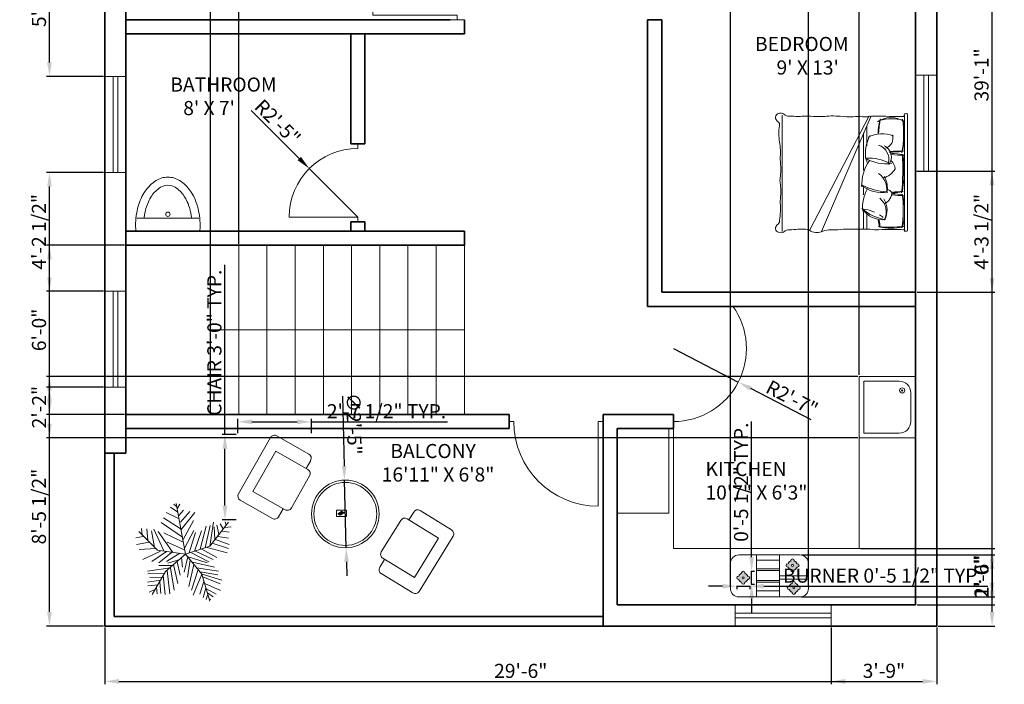
# Model space of a CAD drawing. Units: inches. Extents: x 88375 to 88815, y 24230 to 25146.
# Tile 1 of 3: x 88375 to 88794, y 24230 to 24513. Entities that reach past the tile are written whole.
import ezdxf

# ---------------------------------------------------------------- set-up
doc = ezdxf.new("R2010")
doc.units = ezdxf.units.IN
for name, color, linetype, lineweight in [('A-ANNO-DIMS', 2, 'Continuous', 18), ('A-AREA-IDEN', 7, 'Continuous', 18), ('A-EQPM', 4, 'Continuous', 18), ('A-FLOR-CASE', 7, 'Continuous', 18), ('A-FLOR-STRS', 7, 'Continuous', 18), ('A-WALL', 7, 'Continuous', 35), ('doors', 50, 'Continuous', 18), ('L-PLNT', 7, 'Continuous', 13), ('SANTEH', 5, 'Continuous', 18), ('windows', 70, 'Continuous', 18)]:
    doc.layers.add(name, color=color, linetype=linetype, lineweight=lineweight)
doc.layers.add('A-FURN', color=141, linetype='Continuous', lineweight=18, true_color=0xadddf7)
doc.layers.add('A-FURN-PATT', color=141, linetype='Continuous', lineweight=13, true_color=0xadddf7)
doc.styles.get("Standard").update_dxf_attribs({"font": 'arial.ttf'})
doc.dimstyles.new('ISO-25', dxfattribs={"dimtxt": 6, "dimasz": 6, "dimexe": 1.25, "dimexo": 0.625, "dimtad": 1, "dimdec": 0, "dimlunit": 3, "dimtxsty": 'Standard', "dimcen": 2.5, "dimclrd": 1, "dimclre": 1, "dimclrt": 2, "dimadec": 0, "dimazin": 0, "dimtfac": 1, "dimtdec": 0, "dimtmove": 0, "dimatfit": 3, "dimfxl": 1, "dimarcsym": 0})

# ---------------------------------------------------------------- blocks, each defined once
blk = doc.blocks.new('Trees - Imperial')
for p, q in [((-10.186, 53.64), (-13.084, 55.962)), ((0, 0), (-10.5, 57)), ((-9.099, 51.782), (-6.563, 55.962)), ((-7.288, 39.707), (-21.778, 46.673)), ((-8.737, 47.138), (-17.069, 52.711)), ((-7.65, 43.423), (-2.578, 49.46)), ((-5.839, 35.992), (4.667, 48.067)), ((-5.114, 27.632), (10.463, 46.673)), ((-3.665, 19.273), (-27.574, 35.527)), ((-5.114, 28.097), (-24.676, 40.636)), ((-2.941, 16.486), (8.652, 37.85)), ((27, 9), (48, 36)), ((27.127, 9.056), (31.112, 35.992)), ((38.719, 34.134), (41.979, 28.561)), ((44.153, 36.456), (45.239, 32.741)), ((-31.5, 4.5), (-52.5, 25.5)), ((-48.585, 21.131), (-49.309, 29.026)), ((-43.513, 28.561), (-42.427, 15.558)), ((-38.442, 26.239), (-34.819, 7.663)), ((-35.544, 28.097), (-24.314, 3.947)), ((-14.533, 2.09), (-30.834, 25.31)), ((-24.314, 23.917), (-2.941, 13.7)), ((-1.129, 6.734), (9.014, 26.704)), ((3.942, 1.625), (11.187, 24.381)), ((10.101, 3.483), (17.708, 26.239)), ((16.259, 5.805), (23.142, 31.348)), ((22.055, 7.198), (27.489, 32.277)), ((31.836, 30.883), (32.561, 16.486)), ((35.096, 32.741), (37.27, 22.524)), ((40.53, 25.775), (48.862, 24.846)), ((43.791, 29.954), (51.036, 30.883)), ((-47.498, 19.737), (-55.83, 18.344)), ((-40.615, 13.7), (-55.105, 10.913)), ((-20.691, 13.7), (-1.129, 4.876)), ((29.662, 12.307), (48.137, 6.269)), ((33.285, 16.486), (48.862, 10.913)), ((36.183, 19.737), (48.137, 17.88)), ((-33.37, 6.269), (-52.207, 5.34)), ((-28.299, 3.483), (-47.86, -5.805)), ((-21.416, 3.018), (-38.079, -8.128)), ((0, 0), (-31.5, 4.5)), ((-15.982, 2.09), (-30.11, -9.521)), ((0, 0), (-22.5, -19.5)), ((-6.563, 1.161), (-21.416, -8.128)), ((0, 0), (27, 9)), ((0, 0), (18, -22.5)), ((6.478, 1.625), (26.04, -8.592)), ((11.187, 3.483), (30.749, -5.805)), ((18.07, 5.805), (35.096, -3.483)), ((24.229, 7.663), (46.688, 1.625)), ((-6.563, -5.805), (-19.967, -9.985)), ((-9.461, -8.592), (-6.201, -23.453)), ((-4.752, -3.483), (-3.665, -14.629)), ((2.493, -3.019), (-1.491, -20.202)), ((1.769, -2.555), (24.229, -9.521)), ((5.029, -6.27), (2.131, -25.775)), ((7.565, -9.056), (32.198, -14.629)), ((-17.431, -15.094), (-42.789, -18.809)), ((-24.314, -21.596), (-42.427, -22.06)), ((-22.5, -19.5), (-37.5, -45)), ((-15.257, -12.772), (-30.11, -12.772)), ((-20.691, -18.345), (-17.793, -44.352)), ((-17.069, -15.094), (-12.721, -40.172)), ((-13.446, -11.378), (-8.737, -32.741)), ((9.014, -11.378), (3.58, -35.992)), ((14.085, -16.951), (6.478, -40.172)), ((12.274, -15.094), (36.907, -18.809)), ((16.259, -19.738), (36.183, -22.989)), ((-28.299, -29.026), (-42.789, -31.348)), ((-26.849, -26.24), (-40.253, -25.775)), ((-29.023, -30.884), (-27.936, -43.887)), ((-25.038, -23.918), (-22.865, -45.281)), ((18.07, -22.524), (8.289, -45.745)), ((20.244, -30.419), (15.897, -44.816)), ((18, -22.5), (27, -52.5)), ((18.433, -22.524), (40.53, -29.026)), ((19.157, -25.311), (38.719, -33.206)), ((21.331, -32.741), (39.081, -40.636)), ((-30.834, -34.135), (-42.427, -35.528)), ((-34.457, -39.708), (-40.978, -42.494)), ((-32.646, -36.921), (-31.921, -44.352)), ((22.78, -37.85), (19.519, -48.532)), ((22.78, -38.314), (34.372, -44.816)), ((24.591, -43.423), (30.749, -47.603)), ((24.591, -45.745), (23.142, -50.854)), ((26.764, -49.925), (28.213, -50.854))]:
    blk.add_line(p, q)
blk = doc.blocks.new('BED-DOUBLE-PLAN')
for p, q in [((1.4, 0.9), (1.4, 50.31)), ((15.52, 1.15), (36.6, 50.31)), ((53.33, 0.9), (53.33, 50.31)), ((16.31, 1.15), (41.56, 49.64)), ((17.42, 42.88), (17.42, 49.34)), ((18.75, 41.86), (18.75, 49.34)), ((18.75, 31.74), (18.75, 34.71)), ((18.75, 8.33), (18.75, 24.37)), ((17.42, 19.9), (17.42, 20.88)), ((17.42, 5.64), (17.42, 13.88))]:
    blk.add_line(p, q)
blk.add_lwpolyline([(1.54, 49.41, 0.098699), (1.25, 50.08, 0.222522), (0, 50.08), (0, 0.33, 0.171621), (1.3, 0.3, 0.102495), (1.54, 1.48, 0.015571), (6.35, 1.41, 0.00267), (12.35, 1.29, 0.058958), (15.95, 1.46, -0.038458), (19.2, 1.53, 0.025508), (23.25, 1.53, -0.039412), (28.66, 1.33, 0.016498), (32.6, 1.18, -0.035771), (40.08, 1.43, 0.045388), (45.04, 1.29, -0.080578), (47.62, 1.41, 0.026504), (50.99, 1.23, -0.211134), (52.07, 0.79, 0.329446), (55.35, 0.34, 0.37589), (56.22, 2.29, 0.123892), (55.14, 3.69, -0.342539), (54.6, 5.33, 0.07104), (54.53, 12.17, -0.036442), (54.14, 15.72, -0.046791), (54.19, 18.58, 0.023628), (54.14, 21.2, -0.055897), (54.2, 27.56, 0.053528), (54.38, 28.63, 0.053528), (54.2, 29.69, -0.055897), (54.14, 36.05, 0.026973), (54.19, 38.35, -0.036947), (54.14, 41.97, -0.036442), (54.53, 45.52, -0.281256), (55.14, 47.2, -0.521995), (55.14, 47.2, 0.123892), (56.22, 48.6, 0.37589), (55.35, 50.55, 0.329446), (52.07, 50.1, -0.211134), (50.99, 49.66, 0.026504), (47.62, 49.48, -0.06219), (44.27, 49.36, -0.218233), (41.22, 50.22, 0.123513), (38.6, 50.78, 0.129887), (36.08, 50.23, -0.095063), (32.6, 49.71, 0.016498), (28.66, 49.56, -0.039412), (23.25, 49.36, 0.025508), (19.2, 49.36, -0.038458), (15.95, 49.43, 0.058958), (12.35, 49.6, 0.00267), (6.35, 49.48, 0.015571)], format="xyb", close=True)
for centre, radius, start, end in [((28.69, 41.4), 27.41, 165.0181, 193.7392), ((7.34, -1.74), 50.25, 84.0935, 96.4707), ((54.72, 40.85), 52.84, 171.3714, 186.917), ((6.88, 26.06), 22.91, 77.3175, 101.7435), ((30.71, 48.94), 18.95, 180.6432, 190.2707), ((-1.93, 44.06), 14.51, 5.447, 17.4199), ((17.81, 41.21), 9.06, 151.6404, 211.3345), ((16.4, 41.97), 7.31, 151.8876, 231.8707), ((10.64, 34.91), 10.43, 32.3262, 97), ((7.31, 27.91), 17.47, 47.3201, 81.4624), ((20.44, 56.37), 15.6, 229.9508, 236.951), ((20.44, 56.37), 15.6, 246.2982, 263.8539), ((12.85, 33.14), 6.24, 118.1996, 176.5061), ((2.46, 40.16), 16.73, 330.9467, 5.467), ((2.85, 15.46), 19.59, 79.1667, 93.123), ((2.68, 52.73), 19.37, 267.8261, 281.4767), ((6.96, 53.59), 19.33, 255.3434, 268.3876), ((106.24, 23.67), 104.16, 174.3658, 183.3969), ((7.12, 7.71), 26.2, 91.8337, 100.6945), ((8.83, 34.94), 2.36, 210.1134, 265.8974), ((10.93, 20.25), 13.55, 49.1339, 100.5299), ((18.11, 31.85), 9.49, 168.4081, 212.0077), ((56.67, 24.77), 55.1, 170.934, 187.4266), ((17.21, 32.51), 8.35, 173.5607, 234.2853), ((8.19, 10.11), 23.35, 61.605, 88.1749), ((2.96, 30.11), 16.53, 323.2201, 4.4972), ((12.63, 19.42), 8.48, 105.4018, 149.7122), ((11.01, 24.39), 5.75, 186.8992, 226.0421), ((9.41, 5.14), 16.41, 58.6542, 99.1977), ((12.4, 18.76), 5.47, 144.1671, 243.8421), ((16.24, 36.43), 17.32, 241.0456, 274.1497), ((14.48, 19.78), 6.53, 168.0413, 250.8342), ((2.41, -6.96), 24.84, 79.589, 92.0447), ((43.42, 8.57), 41.72, 168.5485, 188.3029), ((6.97, 44.4), 27.2, 259.5301, 269.934), ((1.41, 17.17), 16.55, 332.3859, 9.8951), ((35.22, 9.22), 33.81, 168.0142, 190.5125), ((1.64, 92.63), 76.52, 270.1063, 274.3312), ((7.34, -22.96), 39.54, 89.1536, 97.5533), ((10.98, 10.47), 4.74, 108.9387, 194.6725), ((10.84, 22.26), 13.47, 249.3026, 296.5026), ((274.44, -22.62), 263.89, 173.2132, 174.5476), ((-20.26, 9.91), 32.87, 348.1169, 357.8849), ((7.08, 12.11), 10.21, 237.51, 303.8336), ((6.79, 19.75), 17.39, 253.9263, 287.1409)]:
    blk.add_arc(centre, radius, start, end)
blk = doc.blocks.new('CHAIR-BALCONY')
for p, q in [((13.87, 34.67), (0.26, 10.71)), ((30.23, 27.65), (16.56, 35.41)), ((6.37, 11.76), (16.1, 28.88)), ((29.8, 21.1), (16.1, 28.88)), ((30.97, 24.96), (29.02, 21.54)), ((22.76, 4.72), (30.53, 18.41)), ((6.37, 11.76), (20.07, 3.98)), ((6.37, 11.76), (20.07, 3.98)), ((14.67, 0.26), (1, 8.02)), ((17.35, 1), (19.3, 4.42))]:
    blk.add_line(p, q)
for centre, start, end in [((15.58, 33.7), 60.3989, 150.3989), ((29.25, 25.94), 330.3989, 60.3989), ((28.82, 19.39), 330.3989, 60.3989), ((1.97, 9.73), 150.3989, 240.3989), ((21.04, 5.69), 240.3989, 330.3989), ((15.64, 1.97), 240.3989, 330.3989)]:
    blk.add_arc(centre, 1.97, start, end)
blk = doc.blocks.new('WINDOW-PLAN-WIDE')
for p, q in [((3.5, 40.79), (3.5, 0)), ((5.5, 40.79), (5.5, 0))]:
    blk.add_line(p, q)
blk.add_lwpolyline([(0, 0), (9, 0), (9, 40.79), (0, 40.79)], close=True)
blk = doc.blocks.new('DOOR-SWING-36IN')
for p, q in [((3, 38), (3, 40)), ((3, 0), (3, 2)), ((3, 2), (39, 2)), ((6, 0), (0, 0))]:
    blk.add_line(p, q)
blk.add_arc((3, 2), 36, 0, 90)
blk = doc.blocks.new('COOKTOP-BURNER')
h = blk.add_hatch(color=256)
h.dxf.hatch_style = 1
h.paths.add_polyline_path([(3.49, 4.67), (3.49, 4.81, 1), (2.04, 4.81), (2.04, 4.67, 0.214506), (0.86, 3.49), (0.72, 3.49, 1), (0.72, 2.04), (0.86, 2.04, 0.214506), (2.04, 0.86), (2.04, 0.72, 1), (3.49, 0.72), (3.49, 0.86, 0.214506), (4.67, 2.04), (4.81, 2.04, 1), (4.81, 3.49), (4.67, 3.49, 0.214506)])
h.paths.add_polyline_path([(3.21, 2.77, -1), (2.32, 2.77, -1)], flags=16)
for p, q in [((2.04, 4.81), (2.04, 4.67)), ((3.49, 4.81), (3.49, 4.67)), ((0.72, 3.49), (0.86, 3.49)), ((0.72, 2.04), (0.86, 2.04)), ((2.04, 0.86), (2.04, 0.72)), ((3.49, 0.86), (3.49, 0.72)), ((4.67, 3.49), (4.81, 3.49)), ((4.67, 2.04), (4.81, 2.04))]:
    blk.add_line(p, q)
blk.add_circle((2.77, 2.77), 0.442)
for centre, radius, start, end in [((2.77, 2.77), 2.04, 110.7864, 159.2136), ((2.77, 4.81), 0.724, 0, 180), ((2.77, 2.77), 2.04, 20.7864, 69.2136), ((0.72, 2.77), 0.724, 90, 270), ((2.77, 2.77), 2.04, 200.7864, 249.2136), ((2.77, 0.72), 0.724, 180, 0), ((2.77, 2.77), 2.04, 290.7864, 339.2136), ((4.81, 2.77), 0.724, 270, 90)]:
    blk.add_arc(centre, radius, start, end)
blk = doc.blocks.new('*D23')
at = {"layer": 'A-ANNO-DIMS', "color": 1, "lineweight": -2, "transparency": 16777216}
for p, q in [((88674.45, 24271.96), (88668.45, 24271.96)), ((88680.45, 24272.16), (88680.45, 24270.71)), ((88680.45, 24271.96), (88685.98, 24271.96)), ((88685.98, 24272.16), (88685.98, 24270.71)), ((88691.98, 24271.96), (88787.24, 24271.96))]:
    blk.add_line(p, q, dxfattribs=at)
at = {"layer": 'A-ANNO-DIMS', "color": 1, "transparency": 16777216}
for points in [[(88674.45, 24272.96), (88674.45, 24270.96), (88680.45, 24271.96)], [(88691.98, 24272.96), (88691.98, 24270.96), (88685.98, 24271.96)]]:
    blk.add_solid(points, dxfattribs=at)
at = {"layer": 'Defpoints', "color": 0, "transparency": 16777216}
for p in [(88680.45, 24272.79), (88685.98, 24272.79), (88685.98, 24271.96)]:
    blk.add_point(p, dxfattribs=at)
at = {"layer": 'A-ANNO-DIMS', "color": 2, "transparency": 16777216, "insert": (88742.61, 24275.69), "char_height": 6, "attachment_point": 5}
blk.add_mtext('BURNER 0\'-5 1/2" TYP.', dxfattribs=at)
blk = doc.blocks.new('*D24')
at = {"layer": 'A-ANNO-DIMS', "color": 1, "lineweight": -2, "transparency": 16777216}
for p, q in [((88686.8, 24284.32), (88686.8, 24342.12)), ((88686.6, 24278.32), (88688.05, 24278.32)), ((88686.8, 24272.79), (88686.8, 24278.32)), ((88686.6, 24272.79), (88688.05, 24272.79)), ((88686.8, 24266.79), (88686.8, 24260.79))]:
    blk.add_line(p, q, dxfattribs=at)
at = {"layer": 'A-ANNO-DIMS', "color": 1, "transparency": 16777216}
for points in [[(88685.8, 24284.32), (88687.8, 24284.32), (88686.8, 24278.32)], [(88685.8, 24266.79), (88687.8, 24266.79), (88686.8, 24272.79)]]:
    blk.add_solid(points, dxfattribs=at)
at = {"layer": 'Defpoints', "color": 0, "transparency": 16777216}
for p in [(88685.98, 24278.32), (88686.8, 24278.32), (88685.98, 24272.79)]:
    blk.add_point(p, dxfattribs=at)
at = {"layer": 'A-ANNO-DIMS', "color": 2, "transparency": 16777216, "insert": (88683.08, 24316.22), "char_height": 6, "attachment_point": 5, "rotation": 90}
blk.add_mtext('0\'-5 1/2" TYP.', dxfattribs=at)
blk = doc.blocks.new('*D27')
at = {"layer": 'A-ANNO-DIMS', "color": 1, "lineweight": -2, "transparency": 16777216}
for p, q in [((88462.68, 24336.49), (88462.68, 24408.65)), ((88467.49, 24336.49), (88461.43, 24336.49)), ((88462.68, 24306.26), (88462.68, 24330.49)), ((88467.49, 24300.26), (88461.43, 24300.26))]:
    blk.add_line(p, q, dxfattribs=at)
at = {"layer": 'A-ANNO-DIMS', "color": 1, "transparency": 16777216}
for points in [[(88461.68, 24330.49), (88463.68, 24330.49), (88462.68, 24336.49)], [(88461.68, 24306.26), (88463.68, 24306.26), (88462.68, 24300.26)]]:
    blk.add_solid(points, dxfattribs=at)
at = {"layer": 'Defpoints', "color": 0, "transparency": 16777216}
for p in [(88462.68, 24336.49), (88468.12, 24336.49), (88468.12, 24300.26)]:
    blk.add_point(p, dxfattribs=at)
at = {"layer": 'A-ANNO-DIMS', "color": 2, "transparency": 16777216, "insert": (88458.95, 24375.57), "char_height": 6, "attachment_point": 5, "rotation": 90}
blk.add_mtext('CHAIR 3\'-0" TYP.', dxfattribs=at)
blk = doc.blocks.new('*D28')
at = {"layer": 'A-ANNO-DIMS', "color": 1, "lineweight": -2, "transparency": 16777216}
for p, q in [((88468.12, 24337.11), (88468.12, 24343.17)), ((88474.12, 24341.92), (88493.47, 24341.92)), ((88499.47, 24337.11), (88499.47, 24343.17)), ((88499.47, 24341.92), (88557.38, 24341.92))]:
    blk.add_line(p, q, dxfattribs=at)
at = {"layer": 'A-ANNO-DIMS', "color": 1, "transparency": 16777216}
for points in [[(88474.12, 24342.92), (88474.12, 24340.92), (88468.12, 24341.92)], [(88493.47, 24342.92), (88493.47, 24340.92), (88499.47, 24341.92)]]:
    blk.add_solid(points, dxfattribs=at)
at = {"layer": 'Defpoints', "color": 0, "transparency": 16777216}
for p in [(88499.47, 24341.92), (88468.12, 24336.49), (88499.47, 24336.49)]:
    blk.add_point(p, dxfattribs=at)
at = {"layer": 'A-ANNO-DIMS', "color": 2, "transparency": 16777216, "insert": (88531.43, 24345.65), "char_height": 6, "attachment_point": 5}
blk.add_mtext('2\'-7 1/2" TYP.', dxfattribs=at)
blk = doc.blocks.new('*D33')
at = {"layer": 'A-ANNO-DIMS', "color": 1, "lineweight": -2, "transparency": 16777216}
for p, q in [((88411.55, 24254.4), (88411.55, 24230.22)), ((88765.55, 24254.4), (88765.55, 24230.22)), ((88417.55, 24231.47), (88759.55, 24231.47))]:
    blk.add_line(p, q, dxfattribs=at)
at = {"layer": 'A-ANNO-DIMS', "color": 1, "transparency": 16777216}
for points in [[(88417.55, 24232.47), (88417.55, 24230.47), (88411.55, 24231.47)], [(88759.55, 24232.47), (88759.55, 24230.47), (88765.55, 24231.47)]]:
    blk.add_solid(points, dxfattribs=at)
at = {"layer": 'Defpoints', "color": 0, "transparency": 16777216}
for p in [(88411.55, 24255.02), (88765.55, 24255.02), (88765.55, 24231.47)]:
    blk.add_point(p, dxfattribs=at)
at = {"layer": 'A-ANNO-DIMS', "color": 2, "transparency": 16777216, "insert": (88588.55, 24235.16), "char_height": 6, "attachment_point": 5}
blk.add_mtext('29\'-6"', dxfattribs=at)
blk = doc.blocks.new('*D34')
at = {"layer": 'A-ANNO-DIMS', "color": 1, "lineweight": -2, "transparency": 16777216}
for p, q in [((88766.18, 24724.02), (88790.35, 24724.02)), ((88789.1, 24261.02), (88789.1, 24718.02)), ((88766.18, 24255.02), (88790.35, 24255.02))]:
    blk.add_line(p, q, dxfattribs=at)
at = {"layer": 'A-ANNO-DIMS', "color": 1, "transparency": 16777216}
for points in [[(88788.1, 24718.02), (88790.1, 24718.02), (88789.1, 24724.02)], [(88788.1, 24261.02), (88790.1, 24261.02), (88789.1, 24255.02)]]:
    blk.add_solid(points, dxfattribs=at)
at = {"layer": 'Defpoints', "color": 0, "transparency": 16777216}
for p in [(88765.55, 24724.02), (88789.1, 24724.02), (88765.55, 24255.02)]:
    blk.add_point(p, dxfattribs=at)
at = {"layer": 'A-ANNO-DIMS', "color": 2, "transparency": 16777216, "insert": (88785.41, 24489.52), "char_height": 6, "attachment_point": 5, "rotation": 90}
blk.add_mtext('39\'-1"', dxfattribs=at)
blk = doc.blocks.new('*D37')
at = {"layer": 'A-ANNO-DIMS', "color": 1, "lineweight": -2, "transparency": 16777216}
for p, q in [((88757.18, 24448.59), (88790.35, 24448.59)), ((88789.1, 24403.02), (88789.1, 24442.59)), ((88757.18, 24397.02), (88790.35, 24397.02))]:
    blk.add_line(p, q, dxfattribs=at)
at = {"layer": 'A-ANNO-DIMS', "color": 1, "transparency": 16777216}
for points in [[(88788.1, 24442.59), (88790.1, 24442.59), (88789.1, 24448.59)], [(88788.1, 24403.02), (88790.1, 24403.02), (88789.1, 24397.02)]]:
    blk.add_solid(points, dxfattribs=at)
at = {"layer": 'Defpoints', "color": 0, "transparency": 16777216}
for p in [(88756.55, 24448.59), (88789.1, 24448.59), (88756.55, 24397.02)]:
    blk.add_point(p, dxfattribs=at)
at = {"layer": 'A-ANNO-DIMS', "color": 2, "transparency": 16777216, "insert": (88785.37, 24422.81), "char_height": 6, "attachment_point": 5, "rotation": 90}
blk.add_mtext('4\'-3 1/2"', dxfattribs=at)
blk = doc.blocks.new('*D39')
at = {"layer": 'A-ANNO-DIMS', "color": 1, "lineweight": -2, "transparency": 16777216}
for p, q in [((88410.93, 24356.67), (88386.75, 24356.67)), ((88388, 24261.02), (88388, 24350.67)), ((88410.93, 24255.02), (88386.75, 24255.02))]:
    blk.add_line(p, q, dxfattribs=at)
at = {"layer": 'A-ANNO-DIMS', "color": 1, "transparency": 16777216}
for points in [[(88387, 24350.67), (88389, 24350.67), (88388, 24356.67)], [(88387, 24261.02), (88389, 24261.02), (88388, 24255.02)]]:
    blk.add_solid(points, dxfattribs=at)
at = {"layer": 'Defpoints', "color": 0, "transparency": 16777216}
for p in [(88388, 24356.67), (88411.55, 24356.67), (88411.55, 24255.02)]:
    blk.add_point(p, dxfattribs=at)
at = {"layer": 'A-ANNO-DIMS', "color": 2, "transparency": 16777216, "insert": (88384.28, 24305.85), "char_height": 6, "attachment_point": 5, "rotation": 90}
blk.add_mtext('8\'-5 1/2"', dxfattribs=at)
blk = doc.blocks.new('*D40')
at = {"layer": 'A-ANNO-DIMS', "color": 1, "lineweight": -2, "transparency": 16777216}
for p, q in [((88410.93, 24448.05), (88386.75, 24448.05)), ((88388, 24403.46), (88388, 24442.05)), ((88410.93, 24397.46), (88386.75, 24397.46))]:
    blk.add_line(p, q, dxfattribs=at)
at = {"layer": 'A-ANNO-DIMS', "color": 1, "transparency": 16777216}
for points in [[(88387, 24442.05), (88389, 24442.05), (88388, 24448.05)], [(88387, 24403.46), (88389, 24403.46), (88388, 24397.46)]]:
    blk.add_solid(points, dxfattribs=at)
at = {"layer": 'Defpoints', "color": 0, "transparency": 16777216}
for p in [(88388, 24448.05), (88411.55, 24448.05), (88411.55, 24397.46)]:
    blk.add_point(p, dxfattribs=at)
at = {"layer": 'A-ANNO-DIMS', "color": 2, "transparency": 16777216, "insert": (88384.28, 24422.76), "char_height": 6, "attachment_point": 5, "rotation": 90}
blk.add_mtext('4\'-2 1/2"', dxfattribs=at)
blk = doc.blocks.new('*D41')
at = {"layer": 'A-ANNO-DIMS', "color": 1, "lineweight": -2, "transparency": 16777216}
for p, q in [((88410.93, 24549.01), (88386.75, 24549.01)), ((88388, 24494.84), (88388, 24543.01)), ((88410.93, 24488.84), (88386.75, 24488.84))]:
    blk.add_line(p, q, dxfattribs=at)
at = {"layer": 'A-ANNO-DIMS', "color": 1, "transparency": 16777216}
for points in [[(88387, 24543.01), (88389, 24543.01), (88388, 24549.01)], [(88387, 24494.84), (88389, 24494.84), (88388, 24488.84)]]:
    blk.add_solid(points, dxfattribs=at)
at = {"layer": 'Defpoints', "color": 0, "transparency": 16777216}
for p in [(88388, 24549.01), (88411.55, 24549.01), (88411.55, 24488.84)]:
    blk.add_point(p, dxfattribs=at)
at = {"layer": 'A-ANNO-DIMS', "color": 2, "transparency": 16777216, "insert": (88384.31, 24518.92), "char_height": 6, "attachment_point": 5, "rotation": 90}
blk.add_mtext('5\'-0"', dxfattribs=at)
blk = doc.blocks.new('*D42')
at = {"layer": 'A-ANNO-DIMS', "color": 1, "lineweight": -2, "transparency": 16777216}
for p, q in [((88720.63, 24254.4), (88720.63, 24230.22)), ((88765.55, 24254.4), (88765.55, 24230.22)), ((88726.63, 24231.47), (88759.55, 24231.47))]:
    blk.add_line(p, q, dxfattribs=at)
at = {"layer": 'A-ANNO-DIMS', "color": 1, "transparency": 16777216}
for points in [[(88726.63, 24232.47), (88726.63, 24230.47), (88720.63, 24231.47)], [(88759.55, 24232.47), (88759.55, 24230.47), (88765.55, 24231.47)]]:
    blk.add_solid(points, dxfattribs=at)
at = {"layer": 'Defpoints', "color": 0, "transparency": 16777216}
for p in [(88720.63, 24255.02), (88765.55, 24255.02), (88765.55, 24231.47)]:
    blk.add_point(p, dxfattribs=at)
at = {"layer": 'A-ANNO-DIMS', "color": 2, "transparency": 16777216, "insert": (88743.09, 24235.16), "char_height": 6, "attachment_point": 5}
blk.add_mtext('3\'-9"', dxfattribs=at)
blk = doc.blocks.new('*D43')
at = {"layer": 'A-ANNO-DIMS', "color": 1, "lineweight": -2, "transparency": 16777216}
for p, q in [((88420.55, 24345.65), (88420.55, 24748.82)), ((88426.55, 24747.57), (88450.55, 24747.57)), ((88456.55, 24345.65), (88456.55, 24748.82))]:
    blk.add_line(p, q, dxfattribs=at)
at = {"layer": 'A-ANNO-DIMS', "color": 1, "transparency": 16777216}
for points in [[(88426.55, 24748.57), (88426.55, 24746.57), (88420.55, 24747.57)], [(88450.55, 24748.57), (88450.55, 24746.57), (88456.55, 24747.57)]]:
    blk.add_solid(points, dxfattribs=at)
at = {"layer": 'Defpoints', "color": 0, "transparency": 16777216}
for p in [(88456.55, 24747.57), (88420.55, 24345.02), (88456.55, 24345.02)]:
    blk.add_point(p, dxfattribs=at)
at = {"layer": 'A-ANNO-DIMS', "color": 2, "transparency": 16777216, "insert": (88438.55, 24751.26), "char_height": 6, "attachment_point": 5}
blk.add_mtext('3\'-0"', dxfattribs=at)
blk = doc.blocks.new('*D44')
at = {"layer": 'A-ANNO-DIMS', "color": 1, "lineweight": -2, "transparency": 16777216}
for p, q in [((88419.93, 24417.02), (88386.75, 24417.02)), ((88388, 24351.02), (88388, 24411.02)), ((88419.93, 24345.02), (88386.75, 24345.02))]:
    blk.add_line(p, q, dxfattribs=at)
at = {"layer": 'A-ANNO-DIMS', "color": 1, "transparency": 16777216}
for points in [[(88387, 24411.02), (88389, 24411.02), (88388, 24417.02)], [(88387, 24351.02), (88389, 24351.02), (88388, 24345.02)]]:
    blk.add_solid(points, dxfattribs=at)
at = {"layer": 'Defpoints', "color": 0, "transparency": 16777216}
for p in [(88388, 24417.02), (88420.55, 24417.02), (88420.55, 24345.02)]:
    blk.add_point(p, dxfattribs=at)
at = {"layer": 'A-ANNO-DIMS', "color": 2, "transparency": 16777216, "insert": (88384.31, 24381.02), "char_height": 6, "attachment_point": 5, "rotation": 90}
blk.add_mtext('6\'-0"', dxfattribs=at)
blk = doc.blocks.new('*D45')
at = {"layer": 'A-ANNO-DIMS', "color": 1, "lineweight": -2, "transparency": 16777216}
for p, q in [((88450.55, 24747.57), (88444.55, 24747.57)), ((88456.55, 24417.65), (88456.55, 24748.82)), ((88456.55, 24747.57), (88468.55, 24747.57)), ((88468.55, 24417.65), (88468.55, 24748.82)), ((88474.55, 24747.57), (88497.19, 24747.57))]:
    blk.add_line(p, q, dxfattribs=at)
at = {"layer": 'A-ANNO-DIMS', "color": 1, "transparency": 16777216}
for points in [[(88450.55, 24748.57), (88450.55, 24746.57), (88456.55, 24747.57)], [(88474.55, 24748.57), (88474.55, 24746.57), (88468.55, 24747.57)]]:
    blk.add_solid(points, dxfattribs=at)
at = {"layer": 'Defpoints', "color": 0, "transparency": 16777216}
for p in [(88468.55, 24747.57), (88456.55, 24417.02), (88468.55, 24417.02)]:
    blk.add_point(p, dxfattribs=at)
at = {"layer": 'A-ANNO-DIMS', "color": 2, "transparency": 16777216, "insert": (88488.87, 24751.26), "char_height": 6, "attachment_point": 5}
blk.add_mtext('1\'-0"', dxfattribs=at)
blk = doc.blocks.new('*D47')
at = {"layer": 'A-ANNO-DIMS', "color": 1, "lineweight": -2, "transparency": 16777216}
for p, q in [((88732.55, 24361.84), (88732.55, 24748.82)), ((88738.55, 24747.57), (88750.55, 24747.57)), ((88756.55, 24361.84), (88756.55, 24748.82))]:
    blk.add_line(p, q, dxfattribs=at)
at = {"layer": 'A-ANNO-DIMS', "color": 1, "transparency": 16777216}
for points in [[(88738.55, 24748.57), (88738.55, 24746.57), (88732.55, 24747.57)], [(88750.55, 24748.57), (88750.55, 24746.57), (88756.55, 24747.57)]]:
    blk.add_solid(points, dxfattribs=at)
at = {"layer": 'Defpoints', "color": 0, "transparency": 16777216}
for p in [(88756.55, 24747.57), (88732.55, 24361.22), (88756.55, 24361.22)]:
    blk.add_point(p, dxfattribs=at)
at = {"layer": 'A-ANNO-DIMS', "color": 2, "transparency": 16777216, "insert": (88744.55, 24751.26), "char_height": 6, "attachment_point": 5}
blk.add_mtext('2\'-0"', dxfattribs=at)
blk = doc.blocks.new('*D48')
at = {"layer": 'A-ANNO-DIMS', "color": 1, "lineweight": -2, "transparency": 16777216}
for p, q in [((88731.93, 24361.22), (88386.75, 24361.22)), ((88388, 24341.11), (88388, 24355.22)), ((88731.93, 24335.11), (88386.75, 24335.11))]:
    blk.add_line(p, q, dxfattribs=at)
at = {"layer": 'A-ANNO-DIMS', "color": 1, "transparency": 16777216}
for points in [[(88387, 24355.22), (88389, 24355.22), (88388, 24361.22)], [(88387, 24341.11), (88389, 24341.11), (88388, 24335.11)]]:
    blk.add_solid(points, dxfattribs=at)
at = {"layer": 'Defpoints', "color": 0, "transparency": 16777216}
for p in [(88388, 24361.22), (88732.55, 24361.22), (88732.55, 24335.11)]:
    blk.add_point(p, dxfattribs=at)
at = {"layer": 'A-ANNO-DIMS', "color": 2, "transparency": 16777216, "insert": (88384.37, 24348.16), "char_height": 6, "attachment_point": 5, "rotation": 90}
blk.add_mtext('2\'-2"', dxfattribs=at)
blk = doc.blocks.new('*D49')
at = {"layer": 'A-ANNO-DIMS', "color": 1, "lineweight": -2, "transparency": 16777216}
for p, q in [((88733.18, 24288.02), (88790.35, 24288.02)), ((88789.1, 24282.02), (88789.1, 24270.02)), ((88757.18, 24264.02), (88790.35, 24264.02))]:
    blk.add_line(p, q, dxfattribs=at)
at = {"layer": 'A-ANNO-DIMS', "color": 1, "transparency": 16777216}
for points in [[(88788.1, 24282.02), (88790.1, 24282.02), (88789.1, 24288.02)], [(88788.1, 24270.02), (88790.1, 24270.02), (88789.1, 24264.02)]]:
    blk.add_solid(points, dxfattribs=at)
at = {"layer": 'Defpoints', "color": 0, "transparency": 16777216}
for p in [(88732.55, 24288.02), (88756.55, 24264.02), (88789.1, 24264.02)]:
    blk.add_point(p, dxfattribs=at)
at = {"layer": 'A-ANNO-DIMS', "color": 2, "transparency": 16777216, "insert": (88785.41, 24276.02), "char_height": 6, "attachment_point": 5, "rotation": 90}
blk.add_mtext('2\'-0"', dxfattribs=at)
blk = doc.blocks.new('*D50')
at = {"layer": 'A-ANNO-DIMS', "color": 1, "lineweight": -2, "transparency": 16777216}
for p, q in [((88677.79, 24271.69), (88677.79, 24748.82)), ((88683.79, 24747.57), (88704.98, 24747.57)), ((88710.98, 24271.69), (88710.98, 24748.82))]:
    blk.add_line(p, q, dxfattribs=at)
at = {"layer": 'A-ANNO-DIMS', "color": 1, "transparency": 16777216}
for points in [[(88683.79, 24748.57), (88683.79, 24746.57), (88677.79, 24747.57)], [(88704.98, 24748.57), (88704.98, 24746.57), (88710.98, 24747.57)]]:
    blk.add_solid(points, dxfattribs=at)
at = {"layer": 'Defpoints', "color": 0, "transparency": 16777216}
for p in [(88710.98, 24747.57), (88677.79, 24271.06), (88710.98, 24271.06)]:
    blk.add_point(p, dxfattribs=at)
at = {"layer": 'A-ANNO-DIMS', "color": 2, "transparency": 16777216, "insert": (88694.38, 24751.26), "char_height": 6, "attachment_point": 5}
blk.add_mtext('2\'-9"', dxfattribs=at)
blk = doc.blocks.new('*D51')
at = {"layer": 'A-ANNO-DIMS', "color": 1, "lineweight": -2, "transparency": 16777216}
for p, q in [((88707.99, 24285.26), (88790.35, 24285.26)), ((88789.1, 24273.44), (88789.1, 24279.26)), ((88707.99, 24267.44), (88790.35, 24267.44))]:
    blk.add_line(p, q, dxfattribs=at)
at = {"layer": 'A-ANNO-DIMS', "color": 1, "transparency": 16777216}
for points in [[(88788.1, 24279.26), (88790.1, 24279.26), (88789.1, 24285.26)], [(88788.1, 24273.44), (88790.1, 24273.44), (88789.1, 24267.44)]]:
    blk.add_solid(points, dxfattribs=at)
at = {"layer": 'Defpoints', "color": 0, "transparency": 16777216}
for p in [(88707.36, 24285.26), (88789.1, 24285.26), (88707.36, 24267.44)]:
    blk.add_point(p, dxfattribs=at)
at = {"layer": 'A-ANNO-DIMS', "color": 2, "transparency": 16777216, "insert": (88785.41, 24276.35), "char_height": 6, "attachment_point": 5, "rotation": 90}
blk.add_mtext('1\'-6"', dxfattribs=at)
blk = doc.blocks.new('*D65')
at = {"layer": 'A-ANNO-DIMS', "color": 1, "lineweight": -2, "transparency": 16777216}
for p, q in [((88512.67, 24352.81), (88513.4, 24323.09)), ((88514.26, 24288.35), (88513.55, 24317.09)), ((88514.41, 24282.35), (88514.56, 24276.35))]:
    blk.add_line(p, q, dxfattribs=at)
at = {"layer": 'A-ANNO-DIMS', "color": 1, "transparency": 16777216}
for points in [[(88514.4, 24323.11), (88512.4, 24323.06), (88513.55, 24317.09)], [(88515.41, 24282.37), (88513.41, 24282.32), (88514.26, 24288.35)]]:
    blk.add_solid(points, dxfattribs=at)
at = {"layer": 'Defpoints', "color": 0, "transparency": 16777216}
for p in [(88513.55, 24317.09), (88514.26, 24288.35)]:
    blk.add_point(p, dxfattribs=at)
at = {"layer": 'A-ANNO-DIMS', "color": 2, "transparency": 16777216, "insert": (88516.81, 24341.04), "char_height": 6, "attachment_point": 5, "rotation": 271.4162}
blk.add_mtext('∅2\'-5"', dxfattribs=at)
blk = doc.blocks.new('*D68')
at = {"layer": 'A-ANNO-DIMS', "color": 1, "lineweight": -2, "transparency": 16777216}
for p, q in [((88473.85, 24474.39), (88494.31, 24453.92)), ((88519.21, 24429.02), (88498.55, 24449.68))]:
    blk.add_line(p, q, dxfattribs=at)
at = {"layer": 'A-ANNO-DIMS', "color": 1, "transparency": 16777216}
blk.add_solid([(88495.02, 24454.63), (88493.6, 24453.22), (88498.55, 24449.68)], dxfattribs=at)
at = {"layer": 'Defpoints', "color": 0, "transparency": 16777216}
for p in [(88498.55, 24449.68), (88519.21, 24429.02)]:
    blk.add_point(p, dxfattribs=at)
at = {"layer": 'A-ANNO-DIMS', "color": 2, "transparency": 16777216, "insert": (88484.56, 24468.88), "char_height": 6, "attachment_point": 5, "rotation": 314.9997}
blk.add_mtext('R2\'-5"', dxfattribs=at)
blk = doc.blocks.new('*D69')
at = {"layer": 'A-ANNO-DIMS', "color": 1, "lineweight": -2, "transparency": 16777216}
for p, q in [((88653.55, 24373.05), (88681.12, 24358.82)), ((88712.17, 24342.8), (88686.45, 24356.07))]:
    blk.add_line(p, q, dxfattribs=at)
at = {"layer": 'A-ANNO-DIMS', "color": 1, "transparency": 16777216}
blk.add_solid([(88686.91, 24356.96), (88686, 24355.18), (88681.12, 24358.82)], dxfattribs=at)
at = {"layer": 'Defpoints', "color": 0, "transparency": 16777216}
for p in [(88653.55, 24373.05), (88681.12, 24358.82)]:
    blk.add_point(p, dxfattribs=at)
at = {"layer": 'A-ANNO-DIMS', "color": 2, "transparency": 16777216, "insert": (88703.65, 24351.29), "char_height": 6, "attachment_point": 5, "rotation": 332.7083}
blk.add_mtext('R2\'-7"', dxfattribs=at)

msp = doc.modelspace()

# ---------------------------------------------------------------- hatches: boundary and pattern name
at = {"layer": 'A-FURN-PATT'}
h = msp.add_hatch(dxfattribs=at)
h.set_pattern_fill('ANSI31', color=256, scale=0.082753, angle=-11.058, style=0)
h.set_pattern_definition([(33.942, (-10027.61523, -6762.06877), (-0.1467022024, 0.2179705913), [])])
h.paths.add_polyline_path([(88510.68, 24302.74), (88510.93, 24302.36), (88511.96, 24302.09), (88513.64, 24303.22), (88512.36, 24303.87)])

# ---------------------------------------------------------------- linework, layer by layer
at = {"layer": 'A-EQPM'}
for p, q in [((88681.41, 24285.26), (88707.36, 24285.26)), ((88688.93, 24276.35), (88688.93, 24285.26)), ((88688.93, 24285.26), (88688.93, 24267.44)), ((88698.59, 24285.26), (88698.59, 24267.44)), ((88677.79, 24271.06), (88677.79, 24281.64)), ((88688.93, 24283.03), (88698.59, 24283.03)), ((88710.98, 24281.64), (88710.98, 24271.06)), ((88688.93, 24279.41), (88698.59, 24279.41)), ((88688.93, 24278.69), (88698.59, 24278.69)), ((88688.93, 24274.34), (88698.59, 24274.34)), ((88688.93, 24273.62), (88698.59, 24273.62)), ((88710.98, 24276.35), (88698.59, 24276.35)), ((88698.59, 24274.9), (88710.98, 24274.9)), ((88688.93, 24270), (88698.59, 24270)), ((88707.36, 24267.44), (88681.41, 24267.44))]:
    msp.add_line(p, q, dxfattribs=at)
for centre, start, end in [((88681.41, 24281.64), 90, 180), ((88707.36, 24281.64), 0, 90), ((88681.41, 24271.06), 180, 270), ((88707.36, 24271.06), 270, 0)]:
    msp.add_arc(centre, 3.62, start, end, dxfattribs=at)
at = {"layer": 'A-FLOR-CASE'}
for p, q in [((88732.55, 24288.02), (88732.55, 24361.22)), ((88732.55, 24361.22), (88756.55, 24361.22)), ((88651.55, 24339.02), (88651.55, 24303.02)), ((88653.55, 24339.02), (88653.55, 24315.02)), ((88653.55, 24315.02), (88653.55, 24288.02)), ((88651.55, 24303.02), (88629.55, 24303.02)), ((88653.55, 24288.02), (88756.55, 24288.02)), ((88756.55, 24288.02), (88732.55, 24288.02))]:
    msp.add_line(p, q, dxfattribs=at)
at = {"layer": 'A-FLOR-STRS'}
for p, q in [((88456.55, 24417.02), (88456.55, 24345.02)), ((88468.55, 24417.02), (88468.55, 24345.02)), ((88480.55, 24417.02), (88480.55, 24345.02)), ((88492.55, 24417.02), (88492.55, 24345.02)), ((88504.55, 24417.02), (88504.55, 24345.02)), ((88516.55, 24417.02), (88516.55, 24345.02)), ((88528.55, 24417.02), (88528.55, 24345.02)), ((88540.55, 24417.02), (88540.55, 24345.02)), ((88552.55, 24417.02), (88552.55, 24345.02)), ((88564.55, 24417.02), (88564.55, 24345.02)), ((88564.55, 24381.02), (88456.55, 24381.02))]:
    msp.add_line(p, q, dxfattribs=at)
at = {"layer": 'A-FURN'}
msp.add_lwpolyline([(88510.15, 24301.63), (88514.41, 24301.63), (88514.41, 24304.27), (88510.15, 24304.27)], close=True, dxfattribs=at)
for radius in [14.38, 13.38]:
    msp.add_circle((88513.9, 24302.72), radius, dxfattribs=at)
at = {"layer": 'A-WALL'}
for p, q in [((88411.55, 24339.02), (88411.55, 24724.02)), ((88765.55, 24724.02), (88765.55, 24255.02)), ((88420.55, 24339.02), (88420.55, 24715.02)), ((88756.55, 24715.02), (88756.55, 24264.02)), ((88420.55, 24639.02), (88420.55, 24513.02)), ((88756.55, 24553.02), (88756.55, 24397.02)), ((88420.55, 24513.02), (88558.55, 24513.02)), ((88564.55, 24513.02), (88564.55, 24507.02)), ((88642.55, 24513.02), (88642.55, 24391.02)), ((88642.55, 24513.02), (88648.55, 24513.02)), ((88648.55, 24513.02), (88648.55, 24397.02)), ((88420.55, 24507.02), (88564.55, 24507.02)), ((88516.21, 24507.02), (88516.21, 24460.24)), ((88522.21, 24507.02), (88522.21, 24460.24)), ((88516.21, 24460.24), (88522.21, 24460.24)), ((88516.21, 24423.02), (88516.21, 24427.02)), ((88516.21, 24427.02), (88522.21, 24427.02)), ((88522.21, 24427.02), (88522.21, 24423.02)), ((88420.55, 24423.02), (88564.55, 24423.02)), ((88564.55, 24423.02), (88564.55, 24417.02)), ((88564.55, 24423.02), (88564.55, 24417.02)), ((88420.55, 24417.02), (88564.55, 24417.02)), ((88648.55, 24397.02), (88756.55, 24397.02)), ((88642.55, 24391.02), (88756.55, 24391.02)), ((88756.55, 24391.02), (88756.55, 24264.02)), ((88420.55, 24345.02), (88583.55, 24345.02)), ((88583.55, 24345.02), (88583.55, 24339.02)), ((88623.55, 24345.02), (88653.55, 24345.02)), ((88623.55, 24345.02), (88623.55, 24255.02)), ((88653.55, 24345.02), (88653.55, 24339.02)), ((88411.55, 24339.02), (88411.55, 24255.02)), ((88420.55, 24339.02), (88583.55, 24339.02)), ((88420.55, 24339.02), (88420.55, 24328.51)), ((88629.55, 24339.02), (88629.55, 24264.02)), ((88629.55, 24339.02), (88653.55, 24339.02)), ((88420.55, 24328.51), (88411.55, 24328.51)), ((88415.55, 24328.51), (88415.55, 24259.02)), ((88629.55, 24264.02), (88756.55, 24264.02)), ((88415.55, 24259.02), (88623.55, 24259.02)), ((88642.55, 24255.02), (88411.55, 24255.02)), ((88623.55, 24255.02), (88765.55, 24255.02))]:
    msp.add_line(p, q, dxfattribs=at)
at = {"layer": 'doors'}
for p, q in [((88516.21, 24460.24), (88522.21, 24460.24)), ((88519.21, 24460.24), (88519.21, 24458.24)), ((88519.21, 24429.02), (88490, 24429.02)), ((88519.21, 24427.02), (88519.21, 24429.02)), ((88516.21, 24427.02), (88522.21, 24427.02))]:
    msp.add_line(p, q, dxfattribs=at)
for centre, radius, start, end in [((88519.21, 24429.02), 29.21, 90, 180), ((88653.55, 24373.05), 31.02, 270, 35.4146)]:
    msp.add_arc(centre, radius, start, end, dxfattribs=at)
at = {"layer": 'SANTEH'}
for p, q in [((88451.6, 24428.52), (88425.15, 24428.52)), ((88452, 24423.02), (88424.75, 24423.02)), ((88734.55, 24359.22), (88749.55, 24359.22)), ((88734.55, 24337.11), (88734.55, 24359.22)), ((88754.55, 24354.22), (88754.55, 24342.11)), ((88749.55, 24337.11), (88734.55, 24337.11))]:
    msp.add_line(p, q, dxfattribs=at)
for points in [[(88438.38, 24446.02, 0.139889), (88433.45, 24444.62, 0.107118), (88428.67, 24440, 0.079812), (88425.77, 24433.63, 0.067459), (88424.66, 24425.44, 0.019694), (88424.75, 24423.02, 0.020439)], [(88452, 24423.02, 0.019694), (88452.1, 24425.44, 0.067459), (88450.99, 24433.63, 0.079812), (88448.08, 24440, 0.107118), (88443.31, 24444.62, 0.139889), (88438.38, 24446.02, 0.139889)], [(88438.38, 24442.59, 0.139889), (88435.26, 24441.7, 0.107118), (88431.53, 24438.09, 0.079812), (88429.07, 24432.72, 0.036069), (88428.3, 24428.86, 0.022172)], [(88448.45, 24428.86, 0.036069), (88447.68, 24432.72, 0.079812), (88445.22, 24438.09, 0.107118), (88441.5, 24441.7, 0.139889), (88438.38, 24442.59, 0.139889)]]:
    msp.add_lwpolyline(points, format="xyb", dxfattribs=at)
msp.add_lwpolyline([(88732.55, 24361.22), (88756.55, 24361.22), (88756.55, 24335.11), (88732.55, 24335.11)], close=True, dxfattribs=at)
for centre, radius in [((88438.38, 24430.25), 0.932), ((88750.87, 24355.25), 1.11), ((88750.87, 24355.25), 0.256)]:
    msp.add_circle(centre, radius, dxfattribs=at)
for centre, start, end in [((88749.55, 24354.22), 0, 90), ((88749.55, 24342.11), 270, 0)]:
    msp.add_arc(centre, 5, start, end, dxfattribs=at)

# ---------------------------------------------------------------- block references
at = {"layer": 'A-EQPM'}
for p in [(88701.43, 24278.06), (88680.45, 24272.79), (88701.95, 24268.47)]:
    msp.add_blockref('COOKTOP-BURNER', p, dxfattribs=at)
at = {"layer": 'A-FURN', "rotation": 180}
msp.add_blockref('BED-DOUBLE-PLAN', (88753.19, 24473.26), dxfattribs=at)
at = {"layer": 'A-FURN'}
msp.add_blockref('CHAIR-BALCONY', (88468.18, 24300.54), dxfattribs=at)
at = {"layer": 'A-FURN', "extrusion": (0, 0, -1), "zscale": -1, "rotation": 61.16139631282593}
msp.add_blockref('CHAIR-BALCONY', (-88536.06, 24264.36), dxfattribs=at)
at = {"layer": 'doors', "extrusion": (0, 0, -1), "zscale": -1}
msp.add_blockref('DOOR-SWING-36IN', (-88564.55, 24513.02), dxfattribs=at)
at = {"layer": 'doors', "extrusion": (0, 0, -1), "zscale": -1, "rotation": 270.0000000000153}
msp.add_blockref('DOOR-SWING-36IN', (-88623.55, 24345.02), dxfattribs=at)
at = {"layer": 'L-PLNT', "xscale": 0.3796093072858473, "yscale": 0.3796093072858473, "zscale": 0.3796093072858473}
msp.add_blockref('Trees - Imperial', (88445.95, 24285.57), dxfattribs=at)
at = {"layer": 'windows'}
for p in [(88411.55, 24448.05), (88756.55, 24448.59), (88411.55, 24356.67)]:
    msp.add_blockref('WINDOW-PLAN-WIDE', p, dxfattribs=at)
at = {"layer": 'windows', "rotation": 269.9999999999687}
msp.add_blockref('WINDOW-PLAN-WIDE', (88679.84, 24264.02), dxfattribs=at)

# ---------------------------------------------------------------- texts
at = {"layer": 'A-AREA-IDEN', "char_height": 6, "attachment_point": 1}
for s, width, insert in [("{\\fArial|b1|i0|c0|p34;  BEDROOM\\P       9' X 13'}", 66.2088, (88684.56, 24505.69)), ("{\\fArial|b1|i0|c0|p34;BATHROOM\\P   8' X 7'}", 48.2457, (88439.42, 24488.43)), ('{\\fArial|b1|i0|c0|p34;   BALCONY\\P 16\'11" X 6\'8"}', 66.2088, (88527.56, 24332.49)), ('{\\fArial|b1|i0|c0|p34;KITCHEN\\P10\'7" X 6\'3"}', 66.2088, (88667.16, 24324.84))]:
    msp.add_mtext_dynamic_manual_height_columns(s, width=width, gutter_width=12.5, heights=[0], dxfattribs=dict(at, insert=insert))

# ---------------------------------------------------------------- dimensions: what is measured, and where the dimension line sits
at = {"layer": 'A-ANNO-DIMS'}
for base, p1, p2, picture, middle in [((88456.55, 24747.57), (88420.55, 24345.02), (88456.55, 24345.02), '*D43', (88438.55, 24751.26)), ((88468.55, 24747.57), (88456.55, 24417.02), (88468.55, 24417.02), '*D45', (88488.87, 24751.26)), ((88710.98, 24747.57), (88677.79, 24271.06), (88710.98, 24271.06), '*D50', (88694.38, 24751.26)), ((88756.55, 24747.57), (88732.55, 24361.22), (88756.55, 24361.22), '*D47', (88744.55, 24751.26)), ((88765.55, 24231.47), (88411.55, 24255.02), (88765.55, 24255.02), '*D33', (88588.55, 24235.16)), ((88765.55, 24231.47), (88720.63, 24255.02), (88765.55, 24255.02), '*D42', (88743.09, 24235.16))]:
    dim = msp.add_linear_dim(base=base, p1=p1, p2=p2, dimstyle='ISO-25', override={"dimdec": 1, "dimlfac": 1, "dimrnd": 0, "dimzin": 1, "dimdsep": 46, "dimlunit": 4, "dimfrac": 2}, dxfattribs=at)
    dim.commit()
    dim.dimension.update_dxf_attribs({"geometry": picture, "text_midpoint": middle})
for base, p1, p2, picture, middle in [((88789.1, 24724.02), (88765.55, 24255.02), (88765.55, 24724.02), '*D34', (88785.41, 24489.52)), ((88388, 24549.01), (88411.55, 24488.84), (88411.55, 24549.01), '*D41', (88384.31, 24518.92)), ((88789.1, 24448.59), (88756.55, 24397.02), (88756.55, 24448.59), '*D37', (88785.37, 24422.81)), ((88388, 24448.05), (88411.55, 24397.46), (88411.55, 24448.05), '*D40', (88384.28, 24422.76)), ((88388, 24417.02), (88420.55, 24345.02), (88420.55, 24417.02), '*D44', (88384.31, 24381.02)), ((88388, 24361.22), (88732.55, 24335.11), (88732.55, 24361.22), '*D48', (88384.37, 24348.16)), ((88388.0025, 24356.6747), (88411.5525, 24255.024), (88411.5525, 24356.6747), '*D39', (88384.2752, 24305.8493)), ((88789.1, 24285.26), (88707.36, 24267.44), (88707.36, 24285.26), '*D51', (88785.41, 24276.35)), ((88789.1, 24264.02), (88732.55, 24288.02), (88756.55, 24264.02), '*D49', (88785.41, 24276.02))]:
    dim = msp.add_linear_dim(base=base, p1=p1, p2=p2, angle=90, dimstyle='ISO-25', override={"dimdec": 1, "dimlfac": 1, "dimrnd": 0, "dimzin": 1, "dimdsep": 46, "dimlunit": 4, "dimfrac": 2}, dxfattribs=at)
    dim.commit()
    dim.dimension.update_dxf_attribs({"geometry": picture, "text_midpoint": middle})
for center, mpoint, picture, middle in [((88519.21, 24429.02), (88498.55, 24449.68), '*D68', (88484.56, 24468.88)), ((88653.55, 24373.05), (88681.12, 24358.82), '*D69', (88703.65, 24351.29))]:
    dim = msp.add_radius_dim(center=center, mpoint=mpoint, dimstyle='ISO-25', override={"dimdec": 1, "dimlfac": 1, "dimrnd": 0, "dimzin": 1, "dimdsep": 46, "dimlunit": 4, "dimfrac": 2}, dxfattribs=at)
    dim.commit()
    dim.dimension.update_dxf_attribs({"geometry": picture, "text_midpoint": middle})
for base, p1, p2, text, picture, middle in [((88462.68, 24336.49), (88468.12, 24300.26), (88468.12, 24336.49), 'CHAIR <> TYP.', '*D27', (88458.95, 24375.57)), ((88686.8, 24278.32), (88685.98, 24272.79), (88685.98, 24278.32), '<> TYP.', '*D24', (88683.08, 24316.22))]:
    dim = msp.add_linear_dim(base=base, p1=p1, p2=p2, angle=90, text=text, dimstyle='ISO-25', override={"dimdec": 1, "dimlfac": 1, "dimrnd": 0, "dimzin": 1, "dimdsep": 46, "dimlunit": 4, "dimfrac": 2}, dxfattribs=at)
    dim.commit()
    dim.dimension.update_dxf_attribs({"geometry": picture, "text_midpoint": middle})
for base, p1, p2, text, picture, middle in [((88499.4747, 24341.924), (88468.1153, 24336.4893), (88499.4747, 24336.4893), '<> TYP.', '*D28', (88531.4278, 24345.6513)), ((88685.98, 24271.96), (88680.45, 24272.79), (88685.98, 24272.79), 'BURNER <> TYP.', '*D23', (88742.61, 24275.69))]:
    dim = msp.add_linear_dim(base=base, p1=p1, p2=p2, text=text, dimstyle='ISO-25', override={"dimdec": 1, "dimlfac": 1, "dimrnd": 0, "dimzin": 1, "dimdsep": 46, "dimlunit": 4, "dimfrac": 2}, dxfattribs=at)
    dim.commit()
    dim.dimension.update_dxf_attribs({"geometry": picture, "text_midpoint": middle})
dim = msp.add_diameter_dim_2p(p1=(88514.2588, 24288.3473), p2=(88513.5483, 24317.0889), dimstyle='ISO-25', override={"dimdec": 1, "dimlfac": 1, "dimrnd": 0, "dimzin": 1, "dimdsep": 46, "dimlunit": 4, "dimfrac": 2}, dxfattribs=at)
dim.commit()
dim.dimension.update_dxf_attribs({"geometry": '*D65', "text_midpoint": (88512.9585, 24340.9453)})

doc.saveas('drawing.dxf')
